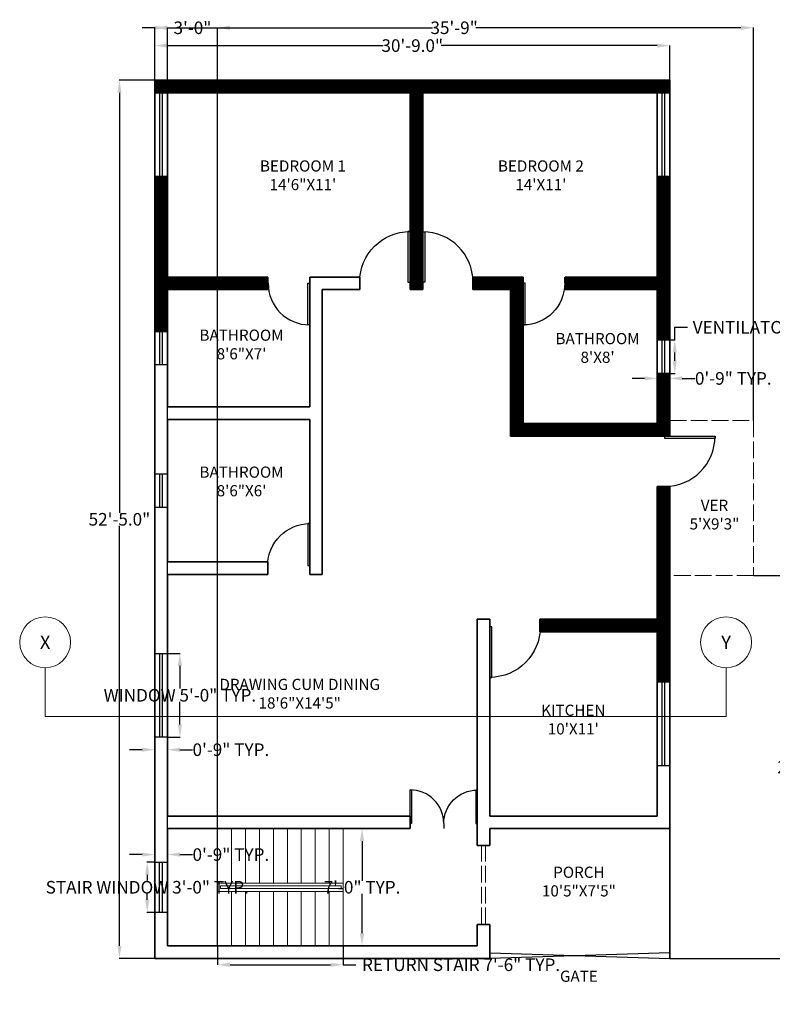
# Model space of a CAD drawing. Units: inches. Extents: x 68 to 1275, y 90 to 1276.
# Tile 2 of 6: x 68 to 608, y 571 to 1276. Entities that reach past the tile are written whole.
import ezdxf

# ---------------------------------------------------------------- set-up
doc = ezdxf.new("R2010")
doc.units = ezdxf.units.IN
doc.header["$MEASUREMENT"] = 0
doc.linetypes.add('ACAD_ISO02W100', pattern=[15, 12, -3])
for name, color, linetype, lineweight in [('A-ANNO-SYMB', 7, 'Continuous', 18), ('A-ANNO-TEXT', 7, 'Continuous', 18), ('A-AREA-IDEN', 7, 'Continuous', 18), ('A-FLOR-OVHD', 8, 'ACAD_ISO02W100', 13), ('A-WALL', 7, 'Continuous', 35), ('A-WALL-PATT', 8, 'Continuous', 13), ('DIM', 2, 'Continuous', 18), ('DOOR', 15, 'Continuous', 25), ('STAIRCASE', 40, 'Continuous', 18), ('WINDOW', 17, 'Continuous', 18)]:
    doc.layers.add(name, color=color, linetype=linetype, lineweight=lineweight)
doc.styles.get("Standard").update_dxf_attribs({"font": 'arial.ttf'})
doc.dimstyles.get("Standard").update_dxf_attribs({"dimtxt": 9, "dimasz": 9, "dimexe": 0.18, "dimexo": 0.0625, "dimgap": 0.09, "dimtad": 0, "dimtih": 1, "dimtoh": 1, "dimdec": 1, "dimzin": 0, "dimdsep": 46, "dimlunit": 3, "dimtxsty": 'Standard', "dimcen": 0.09, "dimadec": 0, "dimazin": 0, "dimtfac": 1, "dimtdec": 1, "dimtofl": 0, "dimtmove": 0, "dimatfit": 3, "dimfxl": 1, "dimtolj": 1, "dimtzin": 0, "dimarcsym": 0})
pattern_1 = [(45, (0, 405.61635), (-0.088388348, 0.088388348), [])]

# ---------------------------------------------------------------- blocks, each defined once
blk = doc.blocks.new('*U2')
for p, q in [((0, 0), (0, -6)), ((40, 0), (40, -6))]:
    blk.add_line(p, q)
blk.add_lwpolyline([(0, 0), (0, 40), (1.75, 40), (1.75, 0)], close=True)
blk.add_arc((0, 0), 40, 0, 90)
blk = doc.blocks.new('W')
at = {"layer": 'DOOR'}
for p, q in [((91.84, 414.95), (100.84, 414.95)), ((91.84, 354.95), (91.84, 414.95)), ((95.34, 354.95), (95.34, 414.95)), ((97.34, 354.95), (97.34, 414.95)), ((100.84, 414.95), (100.84, 354.95)), ((100.84, 354.95), (91.84, 354.95))]:
    blk.add_line(p, q, dxfattribs=at)
blk = doc.blocks.new('V')
at = {"layer": 'DOOR'}
for p, q in [((554.81, 674.59), (563.81, 674.59)), ((554.81, 650.59), (554.81, 674.59)), ((558.31, 650.59), (558.31, 674.59)), ((560.31, 650.59), (560.31, 674.59)), ((563.81, 674.59), (563.81, 650.59)), ((563.81, 650.59), (554.81, 650.59))]:
    blk.add_line(p, q, dxfattribs=at)
blk = doc.blocks.new('W2')
at = {"layer": 'DOOR'}
for p, q in [((130.85, 208.71), (130.85, 244.71)), ((130.85, 244.71), (139.85, 244.71)), ((134.35, 208.71), (134.35, 244.71)), ((136.35, 208.71), (136.35, 244.71)), ((139.85, 244.71), (139.85, 208.71)), ((139.85, 208.71), (130.85, 208.71))]:
    blk.add_line(p, q, dxfattribs=at)
blk = doc.blocks.new('*D7')
at = {"layer": 'Defpoints', "color": 0, "transparency": 16777216}
for p in [(165.19, 1232.47), (139.87, 603.47), (165.19, 603.47)]:
    blk.add_point(p, dxfattribs=at)
at = {"layer": 'DIM', "color": 0, "lineweight": -2, "transparency": 16777216}
for p, q in [((165.13, 1232.47), (139.69, 1232.47)), ((139.87, 1223.47), (139.87, 922.65)), ((139.87, 612.47), (139.87, 913.28)), ((165.13, 603.47), (139.69, 603.47))]:
    blk.add_line(p, q, dxfattribs=at)
at = {"layer": 'DIM', "color": 0, "transparency": 16777216}
for points in [[(138.37, 1223.47), (141.37, 1223.47), (139.87, 1232.47)], [(138.37, 612.47), (141.37, 612.47), (139.87, 603.47)]]:
    blk.add_solid(points, dxfattribs=at)
at = {"layer": 'DIM', "color": 0, "transparency": 16777216, "insert": (139.87, 917.97), "char_height": 9, "attachment_point": 5}
blk.add_mtext('\\A1;52\'-5.0"', dxfattribs=at)
blk = doc.blocks.new('*D8')
at = {"layer": 'Defpoints', "color": 0, "transparency": 16777216}
for p in [(534.19, 1257.2), (165.19, 1232.47), (534.19, 1232.47)]:
    blk.add_point(p, dxfattribs=at)
at = {"layer": 'DIM', "color": 0, "lineweight": -2, "transparency": 16777216}
for p, q in [((165.19, 1232.53), (165.19, 1257.38)), ((174.19, 1257.2), (328.9, 1257.2)), ((525.19, 1257.2), (370.48, 1257.2)), ((534.19, 1232.53), (534.19, 1257.38))]:
    blk.add_line(p, q, dxfattribs=at)
at = {"layer": 'DIM', "color": 0, "transparency": 16777216}
for points in [[(174.19, 1258.7), (174.19, 1255.7), (165.19, 1257.2)], [(525.19, 1258.7), (525.19, 1255.7), (534.19, 1257.2)]]:
    blk.add_solid(points, dxfattribs=at)
at = {"layer": 'DIM', "color": 0, "transparency": 16777216, "insert": (349.69, 1257.2), "char_height": 9, "attachment_point": 5}
blk.add_mtext('\\A1;30\'-9.0"', dxfattribs=at)
blk = doc.blocks.new('STAIR-RETURN-PLAN')
for p, q in [((0, 84), (0, 0)), ((10, 84), (10, 45)), ((20, 84), (20, 45)), ((30, 84), (30, 45)), ((40, 84), (40, 45)), ((50, 84), (50, 45)), ((60, 84), (60, 45)), ((70, 84), (70, 45)), ((80, 84), (80, 45)), ((90, 84), (90, 0)), ((0, 45), (90, 45)), ((2.15, 43), (88.44, 43)), ((2.15, 41), (2.15, 43)), ((88.44, 41), (88.44, 43)), ((0, 39), (90, 39)), ((2.15, 41), (88.44, 41)), ((10, 39), (10, 0)), ((20, 39), (20, 0)), ((30, 39), (30, 0)), ((40, 39), (40, 0)), ((50, 39), (50, 0)), ((60, 39), (60, 0)), ((70, 39), (70, 0)), ((80, 39), (80, 0))]:
    blk.add_line(p, q)
blk = doc.blocks.new('*D47')
at = {"layer": 'Defpoints', "color": 0, "transparency": 16777216}
for p in [(174.19, 821.97), (183.19, 821.97), (174.19, 761.97)]:
    blk.add_point(p, dxfattribs=at)
at = {"layer": 'DIM', "color": 0, "lineweight": -2, "transparency": 16777216}
for p, q in [((174.25, 821.97), (183.37, 821.97)), ((183.19, 812.97), (183.19, 796.72)), ((183.19, 770.97), (183.19, 787.22)), ((174.25, 761.97), (183.37, 761.97))]:
    blk.add_line(p, q, dxfattribs=at)
at = {"layer": 'DIM', "color": 0, "transparency": 16777216}
for points in [[(181.69, 812.97), (184.69, 812.97), (183.19, 821.97)], [(181.69, 770.97), (184.69, 770.97), (183.19, 761.97)]]:
    blk.add_solid(points, dxfattribs=at)
at = {"layer": 'DIM', "color": 0, "transparency": 16777216, "insert": (183.19, 791.97), "char_height": 9, "attachment_point": 5}
blk.add_mtext('\\A1;WINDOW 5\'-0" TYP.', dxfattribs=at)
blk = doc.blocks.new('*D48')
at = {"layer": 'Defpoints', "color": 0, "transparency": 16777216}
for p in [(165.19, 761.97), (174.19, 761.97), (174.19, 752.97)]:
    blk.add_point(p, dxfattribs=at)
at = {"layer": 'DIM', "color": 0, "lineweight": -2, "transparency": 16777216}
for p, q in [((165.19, 761.91), (165.19, 752.79)), ((174.19, 761.91), (174.19, 752.79)), ((156.19, 752.97), (147.19, 752.97)), ((183.19, 752.97), (192.19, 752.97))]:
    blk.add_line(p, q, dxfattribs=at)
at = {"layer": 'DIM', "color": 0, "transparency": 16777216}
for points in [[(156.19, 754.47), (156.19, 751.47), (165.19, 752.97)], [(183.19, 754.47), (183.19, 751.47), (174.19, 752.97)]]:
    blk.add_solid(points, dxfattribs=at)
at = {"layer": 'DIM', "color": 0, "transparency": 16777216, "insert": (219.71, 752.97), "char_height": 9, "attachment_point": 5}
blk.add_mtext('\\A1;0\'-9" TYP.', dxfattribs=at)
blk = doc.blocks.new('*D49')
at = {"layer": 'Defpoints', "color": 0, "transparency": 16777216}
for p in [(534.19, 1046.47), (537.79, 1046.47), (534.19, 1022.47)]:
    blk.add_point(p, dxfattribs=at)
at = {"layer": 'DIM', "color": 0, "lineweight": -2, "transparency": 16777216}
for p, q in [((537.79, 1046.47), (537.79, 1055.47)), ((537.79, 1055.47), (546.79, 1055.47)), ((534.25, 1046.47), (537.97, 1046.47)), ((537.79, 1031.47), (537.79, 1037.47)), ((534.25, 1022.47), (537.97, 1022.47))]:
    blk.add_line(p, q, dxfattribs=at)
at = {"layer": 'DIM', "color": 0, "transparency": 16777216}
for points in [[(536.29, 1037.47), (539.29, 1037.47), (537.79, 1046.47)], [(536.29, 1031.47), (539.29, 1031.47), (537.79, 1022.47)]]:
    blk.add_solid(points, dxfattribs=at)
at = {"layer": 'DIM', "color": 0, "transparency": 16777216, "insert": (615.76, 1055.47), "char_height": 9, "attachment_point": 5}
blk.add_mtext('\\A1;VENTILATOR 2\'-0" TYP.', dxfattribs=at)
blk = doc.blocks.new('*D50')
at = {"layer": 'Defpoints', "color": 0, "transparency": 16777216}
for p in [(525.19, 1022.47), (534.19, 1022.47), (534.19, 1018.87)]:
    blk.add_point(p, dxfattribs=at)
at = {"layer": 'DIM', "color": 0, "lineweight": -2, "transparency": 16777216}
for p, q in [((516.19, 1018.87), (507.19, 1018.87)), ((525.19, 1022.41), (525.19, 1018.69)), ((534.19, 1022.41), (534.19, 1018.69)), ((543.19, 1018.87), (552.19, 1018.87))]:
    blk.add_line(p, q, dxfattribs=at)
at = {"layer": 'DIM', "color": 0, "transparency": 16777216}
for points in [[(516.19, 1020.37), (516.19, 1017.37), (525.19, 1018.87)], [(543.19, 1020.37), (543.19, 1017.37), (534.19, 1018.87)]]:
    blk.add_solid(points, dxfattribs=at)
at = {"layer": 'DIM', "color": 0, "transparency": 16777216, "insert": (579.71, 1018.87), "char_height": 9, "attachment_point": 5}
blk.add_mtext('\\A1;0\'-9" TYP.', dxfattribs=at)
blk = doc.blocks.new('*D51')
at = {"layer": 'Defpoints', "color": 0, "transparency": 16777216}
for p in [(159.79, 672.47), (165.19, 672.47), (165.19, 636.47)]:
    blk.add_point(p, dxfattribs=at)
at = {"layer": 'DIM', "color": 0, "lineweight": -2, "transparency": 16777216}
for p, q in [((165.13, 672.47), (159.61, 672.47)), ((159.79, 663.47), (159.79, 659.22)), ((159.79, 645.47), (159.79, 649.72)), ((165.13, 636.47), (159.61, 636.47))]:
    blk.add_line(p, q, dxfattribs=at)
at = {"layer": 'DIM', "color": 0, "transparency": 16777216}
for points in [[(158.29, 663.47), (161.29, 663.47), (159.79, 672.47)], [(158.29, 645.47), (161.29, 645.47), (159.79, 636.47)]]:
    blk.add_solid(points, dxfattribs=at)
at = {"layer": 'DIM', "color": 0, "transparency": 16777216, "insert": (159.79, 654.47), "char_height": 9, "attachment_point": 5}
blk.add_mtext('\\A1;STAIR WINDOW 3\'-0" TYP.', dxfattribs=at)
blk = doc.blocks.new('*D52')
at = {"layer": 'Defpoints', "color": 0, "transparency": 16777216}
for p in [(174.19, 677.87), (165.19, 672.47), (174.19, 672.47)]:
    blk.add_point(p, dxfattribs=at)
at = {"layer": 'DIM', "color": 0, "lineweight": -2, "transparency": 16777216}
for p, q in [((156.19, 677.87), (147.19, 677.87)), ((165.19, 672.53), (165.19, 678.05)), ((174.19, 672.53), (174.19, 678.05)), ((183.19, 677.87), (192.19, 677.87))]:
    blk.add_line(p, q, dxfattribs=at)
at = {"layer": 'DIM', "color": 0, "transparency": 16777216}
for points in [[(156.19, 679.37), (156.19, 676.37), (165.19, 677.87)], [(183.19, 679.37), (183.19, 676.37), (174.19, 677.87)]]:
    blk.add_solid(points, dxfattribs=at)
at = {"layer": 'DIM', "color": 0, "transparency": 16777216, "insert": (219.71, 677.87), "char_height": 9, "attachment_point": 5}
blk.add_mtext('\\A1;0\'-9" TYP.', dxfattribs=at)
blk = doc.blocks.new('*D53')
at = {"layer": 'Defpoints', "color": 0, "transparency": 16777216}
for p in [(210.19, 612.47), (300.19, 612.47), (300.19, 598.97)]:
    blk.add_point(p, dxfattribs=at)
at = {"layer": 'DIM', "color": 0, "lineweight": -2, "transparency": 16777216}
for p, q in [((210.19, 612.41), (210.19, 598.79)), ((300.19, 612.41), (300.19, 598.79)), ((219.19, 598.97), (291.19, 598.97)), ((300.19, 598.97), (309.19, 598.97))]:
    blk.add_line(p, q, dxfattribs=at)
at = {"layer": 'DIM', "color": 0, "transparency": 16777216}
for points in [[(219.19, 600.47), (219.19, 597.47), (210.19, 598.97)], [(291.19, 600.47), (291.19, 597.47), (300.19, 598.97)]]:
    blk.add_solid(points, dxfattribs=at)
at = {"layer": 'DIM', "color": 0, "transparency": 16777216, "insert": (384.68, 598.97), "char_height": 9, "attachment_point": 5}
blk.add_mtext('\\A1;RETURN STAIR 7\'-6" TYP.', dxfattribs=at)
blk = doc.blocks.new('*D54')
at = {"layer": 'Defpoints', "color": 0, "transparency": 16777216}
for p in [(300.19, 696.47), (313.69, 696.47), (300.19, 612.47)]:
    blk.add_point(p, dxfattribs=at)
at = {"layer": 'DIM', "color": 0, "lineweight": -2, "transparency": 16777216}
for p, q in [((300.25, 696.47), (313.87, 696.47)), ((313.69, 687.47), (313.69, 659.15)), ((313.69, 621.47), (313.69, 649.78)), ((300.25, 612.47), (313.87, 612.47))]:
    blk.add_line(p, q, dxfattribs=at)
at = {"layer": 'DIM', "color": 0, "transparency": 16777216}
for points in [[(312.19, 687.47), (315.19, 687.47), (313.69, 696.47)], [(312.19, 621.47), (315.19, 621.47), (313.69, 612.47)]]:
    blk.add_solid(points, dxfattribs=at)
at = {"layer": 'DIM', "color": 0, "transparency": 16777216, "insert": (313.69, 654.47), "char_height": 9, "attachment_point": 5}
blk.add_mtext('\\A1;7\'-0" TYP.', dxfattribs=at)
blk = doc.blocks.new('*D83')
at = {"layer": 'Defpoints', "color": 0, "transparency": 16777216}
for p in [(594.19, 1269.97), (165.19, 1232.47), (594.19, 988.68)]:
    blk.add_point(p, dxfattribs=at)
at = {"layer": 'DIM', "color": 0, "lineweight": -2, "transparency": 16777216}
for p, q in [((165.19, 1232.53), (165.19, 1270.15)), ((174.19, 1269.97), (364.15, 1269.97)), ((585.19, 1269.97), (395.24, 1269.97)), ((594.19, 988.74), (594.19, 1270.15))]:
    blk.add_line(p, q, dxfattribs=at)
at = {"layer": 'DIM', "color": 0, "transparency": 16777216}
for points in [[(174.19, 1271.47), (174.19, 1268.47), (165.19, 1269.97)], [(585.19, 1271.47), (585.19, 1268.47), (594.19, 1269.97)]]:
    blk.add_solid(points, dxfattribs=at)
at = {"layer": 'DIM', "color": 0, "transparency": 16777216, "insert": (379.69, 1269.97), "char_height": 9, "attachment_point": 5}
blk.add_mtext('\\A1;35\'-9"', dxfattribs=at)
blk = doc.blocks.new('*D84')
at = {"layer": 'Defpoints', "color": 0, "transparency": 16777216}
for p in [(594.19, 877.68), (631.69, 877.68), (534.19, 603.47)]:
    blk.add_point(p, dxfattribs=at)
at = {"layer": 'DIM', "color": 0, "lineweight": -2, "transparency": 16777216}
for p, q in [((594.25, 877.68), (631.87, 877.68)), ((631.69, 868.68), (631.69, 745.26)), ((631.69, 612.47), (631.69, 735.89)), ((534.25, 603.47), (631.87, 603.47))]:
    blk.add_line(p, q, dxfattribs=at)
at = {"layer": 'DIM', "color": 0, "transparency": 16777216}
for points in [[(630.19, 868.68), (633.19, 868.68), (631.69, 877.68)], [(630.19, 612.47), (633.19, 612.47), (631.69, 603.47)]]:
    blk.add_solid(points, dxfattribs=at)
at = {"layer": 'DIM', "color": 0, "transparency": 16777216, "insert": (631.69, 740.57), "char_height": 9, "attachment_point": 5}
blk.add_mtext('\\A1;22\'-10"', dxfattribs=at)
blk = doc.blocks.new('*D85')
at = {"layer": 'Defpoints', "color": 0, "transparency": 16777216}
for p in [(210.192058, 1269.968609), (174.192058, 612.468609), (210.192058, 612.468609)]:
    blk.add_point(p, dxfattribs=at)
at = {"layer": 'DIM', "color": 0, "lineweight": -2, "transparency": 16777216}
for p, q in [((165.192058, 1269.968609), (156.192058, 1269.968609)), ((174.192058, 612.531109), (174.192058, 1270.148609)), ((210.192058, 612.531109), (210.192058, 1270.148609)), ((219.192058, 1269.968609), (228.192058, 1269.968609))]:
    blk.add_line(p, q, dxfattribs=at)
at = {"layer": 'DIM', "color": 0, "transparency": 16777216}
for points in [[(165.192058, 1271.468609), (165.192058, 1268.468609), (174.192058, 1269.968609)], [(219.192058, 1271.468609), (219.192058, 1268.468609), (210.192058, 1269.968609)]]:
    blk.add_solid(points, dxfattribs=at)
at = {"layer": 'DIM', "color": 0, "transparency": 16777216, "insert": (192.192058, 1269.968609), "char_height": 9, "attachment_point": 5}
blk.add_mtext('\\A1;3\'-0"', dxfattribs=at)

msp = doc.modelspace()

# ---------------------------------------------------------------- hatches: boundary and pattern name
at = {"layer": 'A-WALL-PATT'}
h = msp.add_hatch(dxfattribs=at)
h.set_pattern_fill('ANSI31', color=256)
h.set_pattern_definition(pattern_1)
h.paths.add_polyline_path([(348.19, 1223.47), (348.19, 1091.47), (348.19, 1087.89), (348.19, 1082.47), (357.19, 1082.47), (357.19, 1087.87), (357.19, 1123.89), (357.19, 1223.47), (525.19, 1223.47), (534.19, 1223.47), (534.19, 1232.47), (165.19, 1232.47), (165.19, 1223.47), (174.19, 1223.47)])
h = msp.add_hatch(dxfattribs=at)
h.set_pattern_fill('ANSI31', color=256)
h.set_pattern_definition(pattern_1)
h.paths.add_polyline_path([(165.19, 1052.47), (174.19, 1052.47), (174.19, 1082.47), (246.19, 1082.47), (246.19, 1091.47), (174.19, 1091.47), (174.19, 1163.47), (165.19, 1163.47)])
h = msp.add_hatch(dxfattribs=at)
h.set_pattern_fill('ANSI31', color=256)
h.set_pattern_definition(pattern_1)
h.paths.add_polyline_path([(525.19, 1091.47), (459.19, 1091.47), (459.19, 1082.47), (525.19, 1082.47), (525.19, 1046.47), (534.19, 1046.47), (534.19, 1163.47), (525.19, 1163.47)])
h = msp.add_hatch(dxfattribs=at)
h.set_pattern_fill('ANSI31', color=256)
h.set_pattern_definition(pattern_1)
h.paths.add_polyline_path([(429.19, 1087), (429.19, 1091.47), (393.19, 1091.47), (393.19, 1088.9, -0.007125), (393.21, 1087.87), (393.21, 1082.47), (420.19, 1082.47), (420.19, 977.47), (525.19, 977.47), (530.6, 977.47), (534.19, 977.47), (534.19, 1022.47), (525.19, 1022.47), (525.19, 986.47), (429.19, 986.47), (429.19, 1082.47)])
h = msp.add_hatch(dxfattribs=at)
h.set_pattern_fill('ANSI31', color=256)
h.set_pattern_definition(pattern_1)
h.paths.add_polyline_path([(534.19, 941.47), (531.97, 941.47, -0.009518), (530.6, 941.44), (525.19, 941.44), (525.19, 846.47), (441.43, 846.47), (441.43, 841.03, -0.024628), (441.26, 837.47), (525.19, 837.47), (525.19, 801.47), (534.19, 801.47)])

# ---------------------------------------------------------------- linework, layer by layer
at = {"layer": 'A-ANNO-SYMB'}
for p, q in [((86.63, 811.64), (86.63, 776.63)), ((574.56, 776.63), (574.56, 811.64)), ((86.63, 776.63), (574.56, 776.63))]:
    msp.add_line(p, q, dxfattribs=at)
for centre in [(86.63, 829.89), (574.56, 829.89)]:
    msp.add_circle(centre, 18.24, dxfattribs=at)
at = {"layer": 'A-FLOR-OVHD'}
for p, q in [((534.19, 988.68), (594.19, 988.68)), ((594.19, 988.68), (594.19, 877.68)), ((594.19, 877.68), (534.19, 877.68)), ((399.19, 627.86), (399.19, 684.31)), ((402.19, 627.86), (402.19, 684.31))]:
    msp.add_line(p, q, dxfattribs=at)
at = {"layer": 'A-WALL'}
for p, q in [((165.19, 1232.47), (534.19, 1232.47)), ((165.19, 1232.47), (165.19, 603.47)), ((534.19, 1232.47), (534.19, 977.47)), ((174.19, 1223.47), (348.19, 1223.47)), ((174.19, 1223.47), (174.19, 1091.47)), ((348.19, 1223.47), (348.19, 1091.47)), ((357.19, 1223.47), (357.19, 1091.47)), ((357.19, 1223.47), (525.19, 1223.47)), ((525.19, 1223.47), (525.19, 1091.47)), ((174.19, 1091.47), (246.19, 1091.47)), ((246.19, 1082.47), (246.19, 1091.47)), ((276.19, 1082.47), (276.19, 1091.47)), ((276.19, 1091.47), (312.19, 1091.47)), ((312.19, 1091.47), (312.19, 1082.47)), ((348.19, 1091.47), (348.19, 1082.47)), ((357.19, 1091.47), (357.19, 1082.47)), ((393.19, 1091.47), (429.19, 1091.47)), ((393.19, 1091.47), (393.19, 1082.47)), ((429.19, 1082.47), (429.19, 1091.47)), ((459.19, 1082.47), (459.19, 1091.47)), ((459.19, 1091.47), (525.19, 1091.47)), ((174.19, 1082.47), (246.19, 1082.47)), ((174.19, 1082.47), (174.19, 998.47)), ((276.19, 1082.47), (276.19, 998.47)), ((285.19, 1082.47), (285.19, 986.47)), ((285.19, 1082.47), (312.19, 1082.47)), ((348.19, 1082.47), (357.19, 1082.47)), ((393.19, 1082.47), (420.19, 1082.47)), ((420.19, 1082.47), (420.19, 977.47)), ((429.19, 1082.47), (429.19, 986.47)), ((459.19, 1082.47), (525.19, 1082.47)), ((525.19, 1082.47), (525.19, 986.47)), ((174.19, 998.47), (276.19, 998.47)), ((174.19, 989.47), (276.19, 989.47)), ((174.19, 989.47), (174.19, 887.47)), ((276.19, 989.47), (276.19, 887.47)), ((285.19, 986.47), (285.19, 878.47)), ((429.19, 986.47), (525.19, 986.47)), ((420.19, 977.47), (525.19, 977.47)), ((525.19, 977.47), (534.19, 977.47)), ((525.19, 941.47), (525.19, 846.47)), ((525.19, 941.47), (534.19, 941.47)), ((534.19, 941.47), (534.19, 696.47)), ((174.19, 887.47), (246.19, 887.47)), ((246.19, 887.47), (246.19, 878.47)), ((276.19, 887.47), (276.19, 878.47)), ((174.19, 878.47), (246.19, 878.47)), ((174.19, 878.47), (174.19, 705.47)), ((276.19, 878.47), (285.19, 878.47)), ((396.19, 846.47), (396.19, 705.47)), ((396.19, 846.47), (405.19, 846.47)), ((405.19, 837.47), (405.19, 846.47)), ((441.19, 837.47), (441.19, 846.47)), ((441.19, 846.47), (525.19, 846.47)), ((405.19, 837.47), (405.19, 705.47)), ((441.19, 837.47), (525.19, 837.47)), ((525.19, 837.47), (525.19, 705.47)), ((174.19, 705.47), (348.19, 705.47)), ((348.19, 696.47), (348.19, 705.47)), ((396.19, 696.47), (396.19, 705.47)), ((405.19, 705.47), (525.19, 705.47)), ((174.19, 696.47), (348.19, 696.47)), ((174.19, 696.47), (174.19, 612.47)), ((396.19, 684.31), (396.19, 696.47)), ((405.19, 696.47), (534.19, 696.47)), ((405.19, 684.31), (405.19, 696.47)), ((534.19, 603.47), (534.19, 696.47)), ((396.19, 684.31), (405.19, 684.31)), ((396.19, 612.47), (396.19, 627.86)), ((405.19, 627.86), (396.19, 627.86)), ((405.19, 603.47), (405.19, 627.86)), ((174.19, 612.47), (396.19, 612.47)), ((165.19, 603.47), (405.19, 603.47))]:
    msp.add_line(p, q, dxfattribs=at)
at = {"layer": 'DOOR'}
for p, q in [((405.19, 607.47), (534.19, 603.47)), ((534.19, 607.47), (405.19, 603.47))]:
    msp.add_line(p, q, dxfattribs=at)

# ---------------------------------------------------------------- block references
for p, xscale, yscale, zscale in [((348.19, 1087.89), -0.9042317685223638, 0.9042317685223638, 0.9042317685223638), ((357.19, 1087.87), 0.9003656315011651, 0.9003656315011651, 0.9003656315011651), ((276.19, 884.85), -0.7506967006010635, 0.7506967006010635, 0.7506967006010635), ((348.19, 700.08), 0.6023265859053817, 0.6023265859053817, 0.6023265859053817), ((396.19, 700.06), -0.5984766186909284, 0.5984766186909284, 0.5984766186909284)]:
    msp.add_blockref('*U2', p, dxfattribs=dict(at, xscale=xscale, yscale=yscale, zscale=zscale))
for p, xscale, yscale, zscale, rotation in [((276.19, 1087), 0.7446475691979791, 0.7446475691979791, 0.7446475691979791, 180), ((429.19, 1087), -0.745134442192182, 0.745134442192182, 0.745134442192182, 180), ((530.6, 977.47), 0.9006526865982184, 0.9006526865982184, 0.9006526865982184, 270), ((405.19, 841.03), -0.9060456833541303, 0.9060456833541303, 0.9060456833541303, 180)]:
    msp.add_blockref('*U2', p, dxfattribs=dict(at, xscale=xscale, yscale=yscale, zscale=zscale, rotation=rotation))
at = {"layer": 'STAIRCASE'}
msp.add_blockref('STAIR-RETURN-PLAN', (210.19, 612.47), dxfattribs=at)
at = {"layer": 'WINDOW'}
for name, p in [('W', (73.36, 808.52)), ('W', (433.36, 808.52)), ('V', (-389.61, 377.88)), ('V', (-29.61, 371.88)), ('V', (-389.61, 275.88)), ('W', (73.36, 407.02)), ('W', (433.36, 386.52)), ('W2', (34.34, 427.75))]:
    msp.add_blockref(name, p, dxfattribs=at)

# ---------------------------------------------------------------- texts
at = {"layer": 'A-ANNO-SYMB', "char_height": 12, "width": 20.3989, "attachment_point": 5}
for s, insert in [('{\\fTimes New Roman|b0|i0|c0|p18;\\H0.8x;X}', (86.63, 829.89)), ('{\\fTimes New Roman|b0|i0|c0|p18;\\H0.8x;Y}', (574.56, 829.89))]:
    msp.add_mtext(s, dxfattribs=dict(at, insert=insert))
at = {"layer": 'A-ANNO-TEXT', "insert": (469.09, 594.74), "char_height": 8, "attachment_point": 2}
msp.add_mtext_dynamic_manual_height_columns('GATE', width=128.8568, gutter_width=1, heights=[0], dxfattribs=at)
at = {"layer": 'A-AREA-IDEN', "char_height": 8, "attachment_point": 2}
for s, insert in [('BEDROOM 1\\P14\'6"X11\'', (271.34, 1175)), ("BEDROOM 2\\P14'X11'", (441.85, 1175)), ('BATHROOM\\P8\'6"X7\'', (227.36, 1053.82)), ("BATHROOM\\P8'X8'", (482.47, 1051.35)), ('BATHROOM\\P8\'6"X6\'', (227.36, 955.76)), ('VER\\P5\'X9\'3"', (566.24, 932)), ('DRAWING CUM DINING\\P18\'6"X14\'5"', (269.04, 803.74)), ("KITCHEN\\P10'X11'", (465.08, 785.22)), ('PORCH\\P10\'5"X7\'5"', (469.09, 669.21))]:
    msp.add_mtext_dynamic_manual_height_columns(s, width=128.8568, gutter_width=1, heights=[0], dxfattribs=dict(at, insert=insert))

# ---------------------------------------------------------------- dimensions: what is measured, and where the dimension line sits
at = {"layer": 'DIM'}
for base, p1, p2, override, picture, middle in [((210.19, 1269.97), (174.19, 612.47), (210.19, 612.47), {"dimdec": 1, "dimlfac": 1, "dimrnd": 0, "dimzin": 1, "dimdsep": 46, "dimlunit": 4, "dimfrac": 2}, '*D85', (192.19, 1269.97)), ((594.19, 1269.97), (165.19, 1232.47), (594.19, 988.68), {"dimdec": 1, "dimlfac": 1, "dimrnd": 0, "dimzin": 1, "dimdsep": 46, "dimlunit": 4, "dimfrac": 2}, '*D83', (379.69, 1269.97)), ((534.19, 1257.2), (165.19, 1232.47), (534.19, 1232.47), {"dimclrd": 0, "dimclre": 0, "dimclrt": 0}, '*D8', (349.69, 1257.2))]:
    dim = msp.add_linear_dim(base=base, p1=p1, p2=p2, dimstyle='Standard', override=override, dxfattribs=at)
    dim.commit()
    dim.dimension.update_dxf_attribs({"geometry": picture, "text_midpoint": middle})
for base, p1, p2, override, picture, middle in [((139.87, 603.47), (165.19, 1232.47), (165.19, 603.47), {"dimclrd": 0, "dimclre": 0, "dimclrt": 0}, '*D7', (139.87, 917.97)), ((631.69, 877.68), (534.19, 603.47), (594.19, 877.68), {"dimdec": 1, "dimlfac": 1, "dimrnd": 0, "dimzin": 1, "dimdsep": 46, "dimlunit": 4, "dimfrac": 2}, '*D84', (631.69, 740.57))]:
    dim = msp.add_linear_dim(base=base, p1=p1, p2=p2, angle=90, dimstyle='Standard', override=override, dxfattribs=at)
    dim.commit()
    dim.dimension.update_dxf_attribs({"geometry": picture, "text_midpoint": middle})
for base, p1, p2, text, picture, middle in [((537.79, 1046.47), (534.19, 1022.47), (534.19, 1046.47), 'VENTILATOR <> TYP.', '*D49', (615.76, 1055.47)), ((183.19, 821.97), (174.19, 761.97), (174.19, 821.97), 'WINDOW <> TYP.', '*D47', (183.19, 791.97)), ((313.69, 696.47), (300.19, 612.47), (300.19, 696.47), '<> TYP.', '*D54', (313.69, 654.47)), ((159.79, 672.47), (165.19, 636.47), (165.19, 672.47), 'STAIR WINDOW <> TYP.', '*D51', (159.79, 654.47))]:
    dim = msp.add_linear_dim(base=base, p1=p1, p2=p2, angle=90, text=text, dimstyle='Standard', override={"dimdec": 1, "dimlfac": 1, "dimrnd": 0, "dimzin": 1, "dimdsep": 46, "dimlunit": 4, "dimfrac": 2}, dxfattribs=at)
    dim.commit()
    dim.dimension.update_dxf_attribs({"geometry": picture, "text_midpoint": middle})
for base, p1, p2, text, picture, middle in [((534.19, 1018.87), (525.19, 1022.47), (534.19, 1022.47), '<> TYP.', '*D50', (579.71, 1018.87)), ((174.19, 752.97), (165.19, 761.97), (174.19, 761.97), '<> TYP.', '*D48', (219.71, 752.97)), ((174.19, 677.87), (165.19, 672.47), (174.19, 672.47), '<> TYP.', '*D52', (219.71, 677.87)), ((300.19, 598.97), (210.19, 612.47), (300.19, 612.47), 'RETURN STAIR <> TYP.', '*D53', (384.68, 598.97))]:
    dim = msp.add_linear_dim(base=base, p1=p1, p2=p2, text=text, dimstyle='Standard', override={"dimdec": 1, "dimlfac": 1, "dimrnd": 0, "dimzin": 1, "dimdsep": 46, "dimlunit": 4, "dimfrac": 2}, dxfattribs=at)
    dim.commit()
    dim.dimension.update_dxf_attribs({"geometry": picture, "text_midpoint": middle})

doc.saveas('drawing.dxf')
